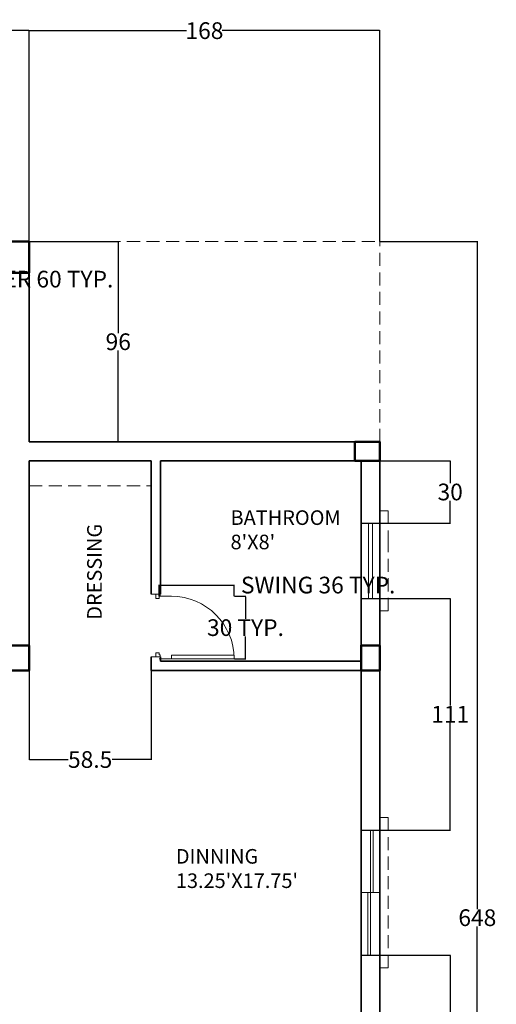
# Model space of a CAD drawing. Units: inches. Extents: x 683 to 1299, y -12 to 932.
# Tile 3 of 3: x 1070 to 1299, y 460 to 932. Entities that reach past the tile are written whole.
import ezdxf

# ---------------------------------------------------------------- set-up
doc = ezdxf.new("R2010")
doc.units = ezdxf.units.IN
doc.header["$LTSCALE"] = 25
doc.header["$MEASUREMENT"] = 0
doc.linetypes.add('HIDDEN', pattern=[0.375, 0.25, -0.125])
for name, color, linetype, lineweight in [('A-ANNO-DIMS', 2, 'Continuous', 18), ('A-AREA-IDEN', 6, 'Continuous', 18), ('A-COLS', 1, 'Continuous', 50), ('A-FLOR-FIXT-HIDN', 8, 'HIDDEN', 13), ('A-GLAZ-OVHD', 7, 'HIDDEN', 13), ('A-ROOF-OVHD', 7, 'HIDDEN', 18), ('A-WALL', 7, 'Continuous', 35)]:
    doc.layers.add(name, color=color, linetype=linetype, lineweight=lineweight)
doc.layers.add('A-DOOR', color=41, linetype='Continuous', lineweight=18, true_color=0xf4ee51)
doc.layers.add('A-GLAZ', color=41, linetype='Continuous', lineweight=18, true_color=0xf4ee51)
doc.styles.get("Standard").update_dxf_attribs({"font": 'arial.ttf'})
doc.dimstyles.get("Standard").update_dxf_attribs({"dimtxt": 8, "dimasz": 0.18, "dimexe": 0.18, "dimexo": 0.0625, "dimgap": 0.09, "dimtad": 0, "dimtih": 1, "dimtoh": 1, "dimdec": 1, "dimzin": 0, "dimdsep": 46, "dimlunit": 3, "dimtxsty": 'Standard', "dimcen": 0.09, "dimadec": 0, "dimazin": 0, "dimtfac": 1, "dimtdec": 1, "dimtofl": 0, "dimtmove": 0, "dimatfit": 3, "dimfxl": 1, "dimtolj": 1, "dimtzin": 0, "dimarcsym": 0})

# ---------------------------------------------------------------- blocks, each defined once
blk = doc.blocks.new('DOOR-SWING-30IN')
for p, q in [((0, 6), (0, 0)), ((30, 6), (30, 0))]:
    blk.add_line(p, q)
blk.add_lwpolyline([(30, 6), (30, 36), (28.25, 36), (28.25, 6)], close=True)
blk.add_arc((30, 6), 30, 90, 180)
blk = doc.blocks.new('DOOR-JAMB-STOP')
for p, q in [((0, 2), (0, 0)), ((0, 2), (1.5, 2)), ((0, 0), (2, 0)), ((1.5, 1), (1.5, 2)), ((2, 1), (1.5, 1)), ((2, 0), (2, 1))]:
    blk.add_line(p, q)
blk = doc.blocks.new('WIN-SLIDER-60IN')
for p, q in [((60, 9), (0, 9)), ((0, 9), (0, 0)), ((30, 9), (30, 0)), ((60, 0), (60, 9)), ((0, 0), (60, 0)), ((30, 0), (60, 0))]:
    blk.add_line(p, q)
for points in [[(30, 4.5), (0, 4.5), (0, 5.76), (30, 5.76)], [(60, 3.24), (30, 3.24), (30, 4.5), (60, 4.5)]]:
    blk.add_lwpolyline(points, close=True)
blk = doc.blocks.new('WIN-36IN')
for p, q in [((36, 9), (0, 9)), ((0, 9), (0, 0)), ((0, 5.5), (36, 5.5)), ((36, 0), (36, 9)), ((0, 3.5), (36, 3.5)), ((0, 0), (36, 0))]:
    blk.add_line(p, q)
blk = doc.blocks.new('COLUMN-12X15IN')
blk.add_lwpolyline([(0, 0), (12, 0), (12, 15), (0, 15)], close=True)
blk = doc.blocks.new('COLUMN-12X9IN')
blk.add_lwpolyline([(0, 9), (0, 0), (12, 0), (12, 9)], close=True)
blk = doc.blocks.new('WIN-HOOD-36IN')
for p, q in [((0, 48), (4, 48)), ((4, 48), (4, 33.44)), ((4, 0), (4, 33.44)), ((0, 0), (4, 0))]:
    blk.add_line(p, q)
blk = doc.blocks.new('*D18')
at = {"layer": 'A-ANNO-DIMS', "color": 0, "lineweight": -2, "ltscale": 25, "transparency": 16777216}
for p, q in [((975.97, 816.54), (975.97, 807.42)), ((1035.97, 816.54), (1035.97, 807.42)), ((976.15, 807.6), (1035.79, 807.6)), ((1035.97, 807.6), (1036.15, 807.6))]:
    blk.add_line(p, q, dxfattribs=at)
at = {"layer": 'A-ANNO-DIMS', "color": 0, "ltscale": 25, "transparency": 16777216}
for points in [[(976.15, 807.63), (976.15, 807.57), (975.97, 807.6)], [(1035.79, 807.63), (1035.79, 807.57), (1035.97, 807.6)]]:
    blk.add_solid(points, dxfattribs=at)
at = {"layer": 'Defpoints', "color": 0, "ltscale": 25, "transparency": 16777216}
for p in [(975.97, 816.6), (1035.97, 816.6), (1035.97, 807.6)]:
    blk.add_point(p, dxfattribs=at)
at = {"layer": 'A-ANNO-DIMS', "color": 0, "ltscale": 25, "transparency": 16777216, "insert": (1077.43, 807.6), "char_height": 8, "attachment_point": 5}
blk.add_mtext('\\A1;SLIDER 60 TYP.', dxfattribs=at)
blk = doc.blocks.new('*D26')
at = {"layer": 'A-ANNO-DIMS', "color": 0, "lineweight": -2, "ltscale": 25, "transparency": 16777216}
for p, q in [((1137.22, 655.66), (1137.22, 661.18)), ((1137.4, 661), (1173.04, 661)), ((1173.22, 655.66), (1173.22, 661.18)), ((1173.22, 661), (1173.4, 661))]:
    blk.add_line(p, q, dxfattribs=at)
at = {"layer": 'A-ANNO-DIMS', "color": 0, "ltscale": 25, "transparency": 16777216}
for points in [[(1137.4, 661.03), (1137.4, 660.97), (1137.22, 661)], [(1173.04, 661.03), (1173.04, 660.97), (1173.22, 661)]]:
    blk.add_solid(points, dxfattribs=at)
at = {"layer": 'Defpoints', "color": 0, "ltscale": 25, "transparency": 16777216}
for p in [(1173.22, 661), (1137.22, 655.6), (1173.22, 655.6)]:
    blk.add_point(p, dxfattribs=at)
at = {"layer": 'A-ANNO-DIMS', "color": 0, "ltscale": 25, "transparency": 16777216, "insert": (1213.43, 661), "char_height": 8, "attachment_point": 5}
blk.add_mtext('\\A1;SWING 36 TYP.', dxfattribs=at)
blk = doc.blocks.new('*D27')
at = {"layer": 'A-ANNO-DIMS', "color": 0, "lineweight": -2, "ltscale": 25, "transparency": 16777216}
for p, q in [((1173.29, 655.6), (1178.8, 655.6)), ((1178.62, 655.42), (1178.62, 644.78)), ((1178.62, 625.78), (1178.62, 636.42)), ((1173.29, 625.6), (1178.8, 625.6))]:
    blk.add_line(p, q, dxfattribs=at)
at = {"layer": 'A-ANNO-DIMS', "color": 0, "ltscale": 25, "transparency": 16777216}
for points in [[(1178.59, 655.42), (1178.65, 655.42), (1178.62, 655.6)], [(1178.59, 625.78), (1178.65, 625.78), (1178.62, 625.6)]]:
    blk.add_solid(points, dxfattribs=at)
at = {"layer": 'Defpoints', "color": 0, "ltscale": 25, "transparency": 16777216}
for p in [(1173.22, 655.6), (1173.22, 625.6), (1178.62, 625.6)]:
    blk.add_point(p, dxfattribs=at)
at = {"layer": 'A-ANNO-DIMS', "color": 0, "ltscale": 25, "transparency": 16777216, "insert": (1178.62, 640.6), "char_height": 8, "attachment_point": 5}
blk.add_mtext('\\A1;30 TYP.', dxfattribs=at)
blk = doc.blocks.new('*D33')
at = {"layer": 'A-ANNO-DIMS', "color": 0, "lineweight": -2, "ltscale": 25, "transparency": 16777216}
for p, q in [((1243.04, 825.6), (1289.85, 825.6)), ((1289.67, 825.42), (1289.67, 505.77)), ((1289.67, 177.78), (1289.67, 497.42)), ((1243.04, 177.6), (1289.85, 177.6))]:
    blk.add_line(p, q, dxfattribs=at)
at = {"layer": 'A-ANNO-DIMS', "color": 0, "ltscale": 25, "transparency": 16777216}
for points in [[(1289.64, 825.42), (1289.7, 825.42), (1289.67, 825.6)], [(1289.64, 177.78), (1289.7, 177.78), (1289.67, 177.6)]]:
    blk.add_solid(points, dxfattribs=at)
at = {"layer": 'Defpoints', "color": 0, "ltscale": 25, "transparency": 16777216}
for p in [(1242.97, 825.6), (1289.67, 825.6), (1242.97, 177.6)]:
    blk.add_point(p, dxfattribs=at)
at = {"layer": 'A-ANNO-DIMS', "color": 0, "ltscale": 25, "transparency": 16777216, "insert": (1289.67, 501.6), "char_height": 8, "attachment_point": 5}
blk.add_mtext('\\A1;648', dxfattribs=at)
blk = doc.blocks.new('*D37')
at = {"layer": 'A-ANNO-DIMS', "color": 0, "lineweight": -2, "ltscale": 25, "transparency": 16777216}
for p, q in [((1035.97, 825.66), (1035.97, 926.85)), ((1036.15, 926.67), (1049.65, 926.67)), ((1074.79, 926.67), (1061.3, 926.67)), ((1074.97, 825.66), (1074.97, 926.85))]:
    blk.add_line(p, q, dxfattribs=at)
at = {"layer": 'A-ANNO-DIMS', "color": 0, "ltscale": 25, "transparency": 16777216}
for points in [[(1036.15, 926.7), (1036.15, 926.64), (1035.97, 926.67)], [(1074.79, 926.7), (1074.79, 926.64), (1074.97, 926.67)]]:
    blk.add_solid(points, dxfattribs=at)
at = {"layer": 'Defpoints', "color": 0, "ltscale": 25, "transparency": 16777216}
for p in [(1074.97, 926.67), (1035.97, 825.6), (1074.97, 825.6)]:
    blk.add_point(p, dxfattribs=at)
at = {"layer": 'A-ANNO-DIMS', "color": 0, "ltscale": 25, "transparency": 16777216, "insert": (1055.47, 926.67), "char_height": 8, "attachment_point": 5}
blk.add_mtext('\\A1;39', dxfattribs=at)
blk = doc.blocks.new('*D38')
at = {"layer": 'A-ANNO-DIMS', "color": 0, "lineweight": -2, "ltscale": 25, "transparency": 16777216}
for p, q in [((1074.97, 825.66), (1074.97, 926.85)), ((1075.15, 926.67), (1150.41, 926.67)), ((1242.79, 926.67), (1167.53, 926.67)), ((1242.97, 825.66), (1242.97, 926.85))]:
    blk.add_line(p, q, dxfattribs=at)
at = {"layer": 'A-ANNO-DIMS', "color": 0, "ltscale": 25, "transparency": 16777216}
for points in [[(1075.15, 926.7), (1075.15, 926.64), (1074.97, 926.67)], [(1242.79, 926.7), (1242.79, 926.64), (1242.97, 926.67)]]:
    blk.add_solid(points, dxfattribs=at)
at = {"layer": 'Defpoints', "color": 0, "ltscale": 25, "transparency": 16777216}
for p in [(1242.97, 926.67), (1074.97, 825.6), (1242.97, 825.6)]:
    blk.add_point(p, dxfattribs=at)
at = {"layer": 'A-ANNO-DIMS', "color": 0, "ltscale": 25, "transparency": 16777216, "insert": (1158.97, 926.67), "char_height": 8, "attachment_point": 5}
blk.add_mtext('\\A1;168', dxfattribs=at)
blk = doc.blocks.new('*D39')
at = {"layer": 'A-ANNO-DIMS', "color": 0, "lineweight": -2, "ltscale": 25, "transparency": 16777216}
for p, q in [((1075.04, 825.6), (1117.85, 825.6)), ((1117.67, 825.42), (1117.67, 781.77)), ((1117.67, 729.78), (1117.67, 773.42)), ((1075.04, 729.6), (1117.85, 729.6))]:
    blk.add_line(p, q, dxfattribs=at)
at = {"layer": 'A-ANNO-DIMS', "color": 0, "ltscale": 25, "transparency": 16777216}
for points in [[(1117.64, 825.42), (1117.7, 825.42), (1117.67, 825.6)], [(1117.64, 729.78), (1117.7, 729.78), (1117.67, 729.6)]]:
    blk.add_solid(points, dxfattribs=at)
at = {"layer": 'Defpoints', "color": 0, "ltscale": 25, "transparency": 16777216}
for p in [(1074.97, 825.6), (1074.97, 729.6), (1117.67, 729.6)]:
    blk.add_point(p, dxfattribs=at)
at = {"layer": 'A-ANNO-DIMS', "color": 0, "ltscale": 25, "transparency": 16777216, "insert": (1117.67, 777.6), "char_height": 8, "attachment_point": 5}
blk.add_mtext('\\A1;96', dxfattribs=at)
blk = doc.blocks.new('*D45')
at = {"layer": 'A-ANNO-DIMS', "color": 0, "lineweight": -2, "ltscale": 25, "transparency": 16777216}
for p, q in [((1234.04, 720.6), (1276.85, 720.6)), ((1276.67, 720.42), (1276.67, 709.78)), ((1276.67, 690.78), (1276.67, 701.42)), ((1234.04, 690.6), (1276.85, 690.6))]:
    blk.add_line(p, q, dxfattribs=at)
at = {"layer": 'A-ANNO-DIMS', "color": 0, "ltscale": 25, "transparency": 16777216}
for points in [[(1276.64, 720.42), (1276.7, 720.42), (1276.67, 720.6)], [(1276.64, 690.78), (1276.7, 690.78), (1276.67, 690.6)]]:
    blk.add_solid(points, dxfattribs=at)
at = {"layer": 'Defpoints', "color": 0, "ltscale": 25, "transparency": 16777216}
for p in [(1233.97, 720.6), (1233.97, 690.6), (1276.67, 690.6)]:
    blk.add_point(p, dxfattribs=at)
at = {"layer": 'A-ANNO-DIMS', "color": 0, "ltscale": 25, "transparency": 16777216, "insert": (1276.67, 705.6), "char_height": 8, "attachment_point": 5}
blk.add_mtext('\\A1;30', dxfattribs=at)
blk = doc.blocks.new('*D46')
at = {"layer": 'A-ANNO-DIMS', "color": 0, "lineweight": -2, "ltscale": 25, "transparency": 16777216}
for p, q in [((1234.04, 654.6), (1276.85, 654.6)), ((1276.67, 654.42), (1276.67, 603.21)), ((1276.67, 543.78), (1276.67, 594.99)), ((1234.04, 543.6), (1276.85, 543.6))]:
    blk.add_line(p, q, dxfattribs=at)
at = {"layer": 'A-ANNO-DIMS', "color": 0, "ltscale": 25, "transparency": 16777216}
for points in [[(1276.64, 654.42), (1276.7, 654.42), (1276.67, 654.6)], [(1276.64, 543.78), (1276.7, 543.78), (1276.67, 543.6)]]:
    blk.add_solid(points, dxfattribs=at)
at = {"layer": 'Defpoints', "color": 0, "ltscale": 25, "transparency": 16777216}
for p in [(1233.97, 654.6), (1233.97, 543.6), (1276.67, 543.6)]:
    blk.add_point(p, dxfattribs=at)
at = {"layer": 'A-ANNO-DIMS', "color": 0, "ltscale": 25, "transparency": 16777216, "insert": (1276.67, 599.1), "char_height": 8, "attachment_point": 5}
blk.add_mtext('\\A1;111', dxfattribs=at)
blk = doc.blocks.new('*D47')
at = {"layer": 'A-ANNO-DIMS', "color": 0, "lineweight": -2, "ltscale": 25, "transparency": 16777216}
for p, q in [((1234.04, 483.6), (1276.85, 483.6)), ((1276.67, 483.42), (1276.67, 439.4)), ((1276.67, 387.03), (1276.67, 431.05)), ((1234.04, 386.85), (1276.85, 386.85))]:
    blk.add_line(p, q, dxfattribs=at)
at = {"layer": 'A-ANNO-DIMS', "color": 0, "ltscale": 25, "transparency": 16777216}
for points in [[(1276.64, 483.42), (1276.7, 483.42), (1276.67, 483.6)], [(1276.64, 387.03), (1276.7, 387.03), (1276.67, 386.85)]]:
    blk.add_solid(points, dxfattribs=at)
at = {"layer": 'Defpoints', "color": 0, "ltscale": 25, "transparency": 16777216}
for p in [(1233.97, 483.6), (1233.97, 386.85), (1276.67, 386.85)]:
    blk.add_point(p, dxfattribs=at)
at = {"layer": 'A-ANNO-DIMS', "color": 0, "ltscale": 25, "transparency": 16777216, "insert": (1276.67, 435.22), "char_height": 8, "attachment_point": 5}
blk.add_mtext('\\A1;96.75', dxfattribs=at)
blk = doc.blocks.new('*D53')
at = {"layer": 'A-ANNO-DIMS', "color": 0, "lineweight": -2, "ltscale": 25, "transparency": 16777216}
for p, q in [((1074.97, 620.04), (1074.97, 577.22)), ((1133.47, 620.04), (1133.47, 577.22)), ((1075.15, 577.4), (1093.71, 577.4)), ((1133.29, 577.4), (1114.73, 577.4))]:
    blk.add_line(p, q, dxfattribs=at)
at = {"layer": 'A-ANNO-DIMS', "color": 0, "ltscale": 25, "transparency": 16777216}
for points in [[(1075.15, 577.43), (1075.15, 577.37), (1074.97, 577.4)], [(1133.29, 577.43), (1133.29, 577.37), (1133.47, 577.4)]]:
    blk.add_solid(points, dxfattribs=at)
at = {"layer": 'Defpoints', "color": 0, "ltscale": 25, "transparency": 16777216}
for p in [(1074.97, 620.1), (1133.47, 620.1), (1074.97, 577.4)]:
    blk.add_point(p, dxfattribs=at)
at = {"layer": 'A-ANNO-DIMS', "color": 0, "ltscale": 25, "transparency": 16777216, "insert": (1104.22, 577.4), "char_height": 8, "attachment_point": 5}
blk.add_mtext('\\A1;58.5', dxfattribs=at)

msp = doc.modelspace()

# ---------------------------------------------------------------- linework, layer by layer
at = {"layer": 'A-COLS'}
for p, q in [((1230.973, 729.599), (1230.973, 720.599)), ((1065.973, 620.099), (1074.973, 620.099)), ((1233.973, 620.099), (1242.973, 620.099))]:
    msp.add_line(p, q, dxfattribs=at)
at = {"layer": 'A-DOOR'}
for p, q in [((1137.973, 656.599), (1133.473, 656.599)), ((1137.973, 626.599), (1133.473, 626.599))]:
    msp.add_line(p, q, dxfattribs=at)
at = {"layer": 'A-FLOR-FIXT-HIDN'}
msp.add_line((1074.973, 708.599), (1133.473, 708.599), dxfattribs=at)
at = {"layer": 'A-GLAZ'}
for p, q in [((1242.973, 690.599), (1242.973, 696.599)), ((1233.973, 672.599), (1233.973, 690.599)), ((1242.973, 654.599), (1242.973, 690.599)), ((1242.973, 654.599), (1242.973, 648.599)), ((1242.973, 543.599), (1242.973, 549.599)), ((1233.973, 513.599), (1233.973, 543.599)), ((1233.973, 543.599), (1242.973, 543.599)), ((1233.973, 483.599), (1233.973, 543.599)), ((1242.973, 543.599), (1242.973, 483.599)), ((1242.973, 483.599), (1233.973, 483.599)), ((1242.973, 483.599), (1242.973, 477.599))]:
    msp.add_line(p, q, dxfattribs=at)
at = {"layer": 'A-GLAZ-OVHD'}
for p, q in [((1242.973, 549.599), (1246.973, 549.599)), ((1246.973, 549.599), (1246.973, 500.352)), ((1246.973, 477.599), (1246.973, 500.352)), ((1242.973, 477.599), (1246.973, 477.599))]:
    msp.add_line(p, q, dxfattribs=at)
at = {"layer": 'A-ROOF-OVHD'}
for p in [(1074.973, 825.599), (1242.973, 729.599)]:
    msp.add_line(p, (1242.973, 825.599), dxfattribs=at)
at = {"layer": 'A-WALL'}
for p, q in [((738.973, 825.599), (1074.973, 825.599)), ((1074.973, 825.599), (1074.973, 729.599)), ((1074.973, 729.599), (1242.973, 729.599)), ((1242.973, 729.599), (1242.973, 177.599)), ((1074.973, 720.599), (1133.473, 720.599)), ((1074.973, 720.599), (1074.973, 620.099)), ((1133.473, 720.599), (1133.473, 656.599)), ((1137.973, 720.599), (1137.973, 656.599)), ((1137.973, 720.599), (1233.973, 720.599)), ((1233.973, 720.599), (1233.973, 624.599)), ((1133.473, 626.599), (1133.473, 620.099)), ((1137.973, 626.599), (1137.973, 624.599)), ((1137.973, 624.599), (1233.973, 624.599)), ((1133.473, 620.099), (1233.973, 620.099)), ((1233.973, 620.099), (1233.973, 407.099))]:
    msp.add_line(p, q, dxfattribs=at)

# ---------------------------------------------------------------- block references
at = {"layer": 'A-COLS'}
msp.add_blockref('COLUMN-12X15IN', (1062.973, 810.599), dxfattribs=at)
for p, rotation in [((1242.973, 729.599), 180), ((1065.973, 632.099), 270.0000000000001), ((1233.973, 632.099), 270.0000000000001)]:
    msp.add_blockref('COLUMN-12X9IN', p, dxfattribs=dict(at, rotation=rotation))
at = {"layer": 'A-DOOR', "extrusion": (0, 0, -1), "zscale": -1, "rotation": 180}
msp.add_blockref('DOOR-JAMB-STOP', (-1135.723, 656.599), dxfattribs=at)
at = {"layer": 'A-DOOR', "rotation": 269.9999999999998}
msp.add_blockref('DOOR-SWING-30IN', (1137.223, 655.599), dxfattribs=at)
at = {"layer": 'A-DOOR'}
msp.add_blockref('DOOR-JAMB-STOP', (1135.723, 626.599), dxfattribs=at)
at = {"layer": 'A-GLAZ'}
for name, p, rotation in [('WIN-36IN', (1242.973, 654.599), 89.99999999999957), ('WIN-SLIDER-60IN', (1233.973, 543.599), 270)]:
    msp.add_blockref(name, p, dxfattribs=dict(at, rotation=rotation))
at = {"layer": 'A-GLAZ-OVHD'}
msp.add_blockref('WIN-HOOD-36IN', (1242.973, 648.599), dxfattribs=at)

# ---------------------------------------------------------------- texts
at = {"layer": 'A-AREA-IDEN', "ltscale": 25, "char_height": 7, "attachment_point": 1}
for s, insert in [("BATHROOM\\P8'X8'", (1171.468, 696.811)), ("DINNING\\P13.25'X17.75'", (1145.286, 534.501))]:
    msp.add_mtext_dynamic_manual_height_columns(s, width=117.16603, gutter_width=1, heights=[0], dxfattribs=dict(at, insert=insert))
at = {"layer": 'A-AREA-IDEN', "ltscale": 25, "insert": (1102.787, 644.398), "char_height": 7, "attachment_point": 1, "rotation": 90}
msp.add_mtext_dynamic_manual_height_columns('DRESSING', width=117.16603, gutter_width=1, heights=[0], dxfattribs=at)

# ---------------------------------------------------------------- dimensions: what is measured, and where the dimension line sits
at = {"layer": 'A-ANNO-DIMS', "ltscale": 25}
for base, p1, p2, picture, middle in [((1074.973, 926.672), (1035.973, 825.599), (1074.973, 825.599), '*D37', (1055.473, 926.672)), ((1242.973, 926.672), (1074.973, 825.599), (1242.973, 825.599), '*D38', (1158.973, 926.672))]:
    dim = msp.add_linear_dim(base=base, p1=p1, p2=p2, dimstyle='Standard', override={"dimdec": 0, "dimlfac": 1, "dimrnd": 0, "dimzin": 0, "dimdsep": 46, "dimlunit": 2}, dxfattribs=at)
    dim.commit()
    dim.dimension.update_dxf_attribs({"geometry": picture, "text_midpoint": middle})
for base, p1, p2, text, picture, middle in [((1035.973, 807.599), (975.973, 816.599), (1035.973, 816.599), 'SLIDER <> TYP.', '*D18', (1077.433, 807.599)), ((1173.223, 660.999), (1137.223, 655.599), (1173.223, 655.599), 'SWING <> TYP.', '*D26', (1213.433, 660.999))]:
    dim = msp.add_linear_dim(base=base, p1=p1, p2=p2, text=text, dimstyle='Standard', override={"dimdec": 0, "dimlfac": 1, "dimrnd": 0, "dimzin": 0, "dimdsep": 46, "dimlunit": 2}, dxfattribs=at)
    dim.commit()
    dim.dimension.update_dxf_attribs({"geometry": picture, "text_midpoint": middle})
for base, p1, p2, angle, override, picture, middle in [((1117.673, 729.599), (1074.973, 825.599), (1074.973, 729.599), 270, {"dimdec": 0, "dimlfac": 1, "dimrnd": 0, "dimzin": 0, "dimdsep": 46, "dimlunit": 2}, '*D39', (1117.673, 777.599)), ((1289.673, 825.599), (1242.973, 177.599), (1242.973, 825.599), 90, {"dimdec": 0, "dimlfac": 1, "dimrnd": 0, "dimzin": 0, "dimdsep": 46, "dimlunit": 2}, '*D33', (1289.673, 501.599)), ((1276.673, 690.599), (1233.973, 720.599), (1233.973, 690.599), 270, {"dimdec": 0, "dimlfac": 1, "dimrnd": 0, "dimzin": 0, "dimdsep": 46, "dimlunit": 2}, '*D45', (1276.673, 705.599)), ((1276.673, 543.599), (1233.973, 654.599), (1233.973, 543.599), 270, {"dimdec": 0, "dimlfac": 1, "dimrnd": 0, "dimzin": 0, "dimdsep": 46, "dimlunit": 2}, '*D46', (1276.673, 599.099)), ((1074.973, 577.399), (1133.473, 620.099), (1074.973, 620.099), 180, {"dimdec": 1, "dimlfac": 1, "dimrnd": 0, "dimzin": 0, "dimdsep": 46, "dimlunit": 2}, '*D53', (1104.223, 577.399)), ((1276.673, 386.849), (1233.973, 483.599), (1233.973, 386.849), 270, {"dimdec": 2, "dimlfac": 1, "dimrnd": 0, "dimzin": 0, "dimdsep": 46, "dimlunit": 2}, '*D47', (1276.673, 435.224))]:
    dim = msp.add_linear_dim(base=base, p1=p1, p2=p2, angle=angle, dimstyle='Standard', override=override, dxfattribs=at)
    dim.commit()
    dim.dimension.update_dxf_attribs({"geometry": picture, "text_midpoint": middle})
dim = msp.add_linear_dim(base=(1178.623, 625.599), p1=(1173.223, 655.599), p2=(1173.223, 625.599), angle=270, text='<> TYP.', dimstyle='Standard', override={"dimdec": 0, "dimlfac": 1, "dimrnd": 0, "dimzin": 0, "dimdsep": 46, "dimlunit": 2}, dxfattribs=at)
dim.commit()
dim.dimension.update_dxf_attribs({"geometry": '*D27', "text_midpoint": (1178.623, 640.599)})

doc.saveas('drawing.dxf')
